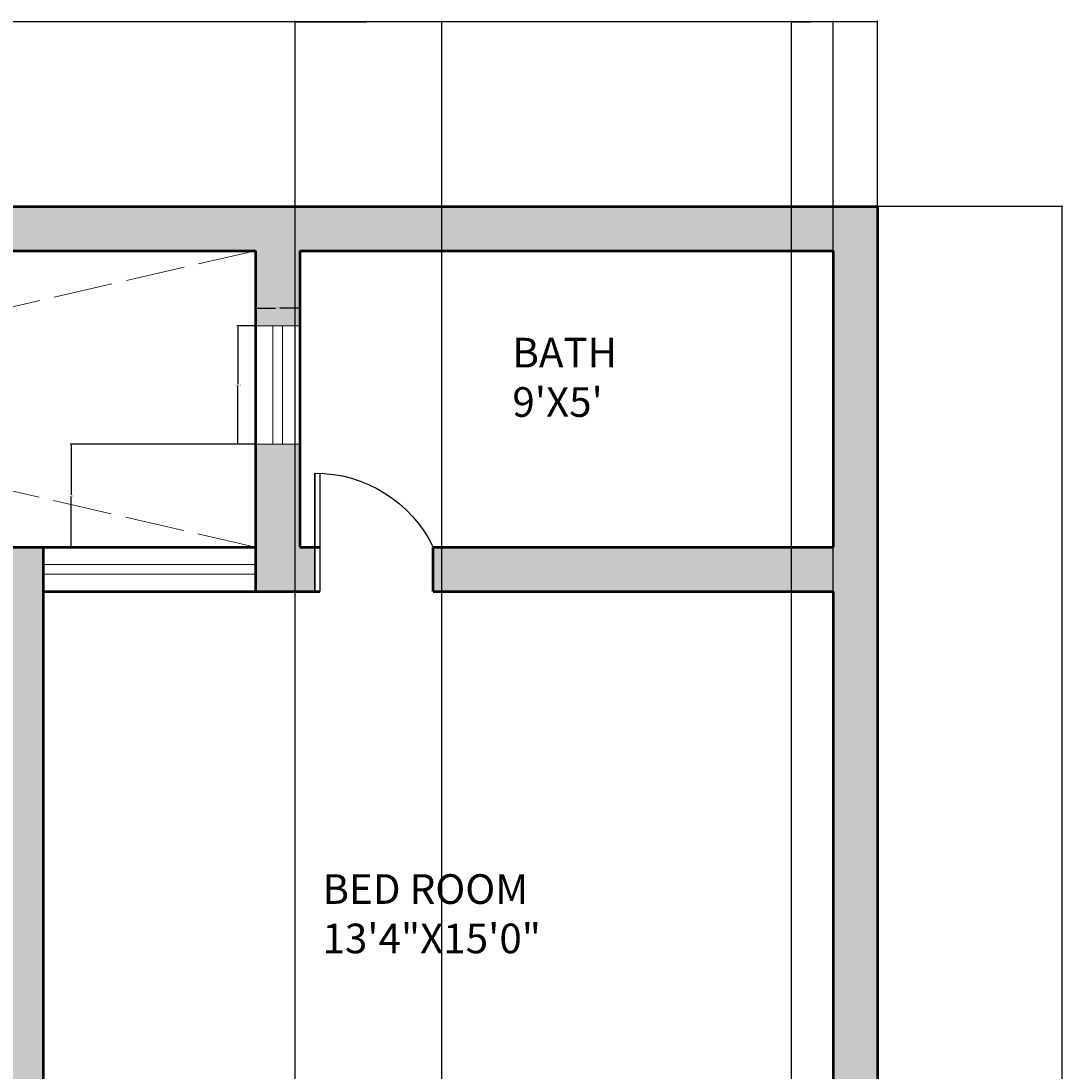
# Model space of a CAD drawing. Units: inches. Extents: x 383 to 970, y 275 to 1088.
# Tile 11 of 11: x 759 to 970, y 875 to 1088. Entities that reach past the tile are written whole.
import ezdxf

# ---------------------------------------------------------------- set-up
doc = ezdxf.new("R2010")
doc.units = ezdxf.units.IN
doc.header["$MEASUREMENT"] = 0
doc.linetypes.add('ACAD_ISO02W100', pattern=[15, 12, -3])
for name, color, linetype, lineweight in [('A-ANNO-DIMS', 2, 'Continuous', 18), ('A-AREA-IDEN', 7, 'Continuous', 18), ('A-DOOR', 3, 'Continuous', 25), ('A-FLOR-OPEN', 8, 'ACAD_ISO02W100', 13), ('A-GLAZ', 4, 'Continuous', 18), ('A-WALL', 7, 'Continuous', 50)]:
    doc.layers.add(name, color=color, linetype=linetype, lineweight=lineweight)
doc.layers.add('A-WALL-PATT', color=251, linetype='Continuous', lineweight=13, true_color=0x636466)
doc.styles.get("Standard").update_dxf_attribs({"font": 'arial.ttf'})
doc.dimstyles.get("Standard").update_dxf_attribs({"dimtxt": 0.18, "dimasz": 0.18, "dimexe": 0.18, "dimexo": 0.0625, "dimgap": 0.09, "dimtad": 0, "dimtih": 1, "dimtoh": 1, "dimdec": 4, "dimzin": 0, "dimdsep": 46, "dimtxsty": 'Standard', "dimcen": 0.09, "dimadec": 0, "dimazin": 0, "dimtfac": 1, "dimtdec": 4, "dimtofl": 0, "dimtmove": 0, "dimatfit": 3, "dimfxl": 1, "dimtolj": 1, "dimtzin": 0, "dimarcsym": 0})

# ---------------------------------------------------------------- blocks, each defined once
blk = doc.blocks.new('DOOR-LEAF-24IN')
for p, q in [((23, 24), (23, 0)), ((24, 0), (24, 24)), ((24, 0), (23, 0))]:
    blk.add_line(p, q)
blk.add_arc((24, -2.7), 26.7, 90, 154.0108)
blk = doc.blocks.new('WIN-VENT-24IN')
for p, q in [((0, 0), (0, 24)), ((3.5, 0), (3.5, 24)), ((5.5, 24), (5.5, 0)), ((9, 24), (9, 0))]:
    blk.add_line(p, q)
blk = doc.blocks.new('WIN-43IN')
for p, q in [((43, 9), (0, 9)), ((43, 5.5), (0, 5.5)), ((0, 3.5), (43, 3.5)), ((0, 0), (43, 0))]:
    blk.add_line(p, q)
blk = doc.blocks.new('*D19')
at = {"layer": 'A-ANNO-DIMS', "color": 0, "lineweight": -2, "transparency": 16777216}
for p, q in [((806.18, 1025.95), (802.46, 1025.95)), ((802.64, 1025.77), (802.64, 1014.13)), ((802.64, 1002.13), (802.64, 1013.77)), ((806.18, 1001.95), (802.46, 1001.95))]:
    blk.add_line(p, q, dxfattribs=at)
at = {"layer": 'A-ANNO-DIMS', "color": 0, "transparency": 16777216}
for points in [[(802.61, 1025.77), (802.67, 1025.77), (802.64, 1025.95)], [(802.61, 1002.13), (802.67, 1002.13), (802.64, 1001.95)]]:
    blk.add_solid(points, dxfattribs=at)
at = {"layer": 'Defpoints', "color": 0, "transparency": 16777216}
for p in [(806.24, 1025.95), (802.64, 1001.95), (806.24, 1001.95)]:
    blk.add_point(p, dxfattribs=at)
at = {"layer": 'A-ANNO-DIMS', "color": 0, "transparency": 16777216, "insert": (802.64, 1013.95), "char_height": 0.18, "attachment_point": 5}
blk.add_mtext('\\A1;VENT 24 TYP.', dxfattribs=at)
blk = doc.blocks.new('*D20')
at = {"layer": 'A-ANNO-DIMS', "color": 0, "lineweight": -2, "transparency": 16777216}
for p, q in [((806.24, 1026.01), (806.24, 1029.73)), ((806.42, 1029.55), (810.28, 1029.55)), ((815.06, 1029.55), (811.2, 1029.55)), ((815.24, 1026.01), (815.24, 1029.73))]:
    blk.add_line(p, q, dxfattribs=at)
at = {"layer": 'A-ANNO-DIMS', "color": 0, "transparency": 16777216}
for points in [[(806.42, 1029.58), (806.42, 1029.52), (806.24, 1029.55)], [(815.06, 1029.58), (815.06, 1029.52), (815.24, 1029.55)]]:
    blk.add_solid(points, dxfattribs=at)
at = {"layer": 'Defpoints', "color": 0, "transparency": 16777216}
for p in [(806.24, 1029.55), (806.24, 1025.95), (815.24, 1025.95)]:
    blk.add_point(p, dxfattribs=at)
at = {"layer": 'A-ANNO-DIMS', "color": 0, "transparency": 16777216, "insert": (810.74, 1029.55), "char_height": 0.18, "attachment_point": 5}
blk.add_mtext('\\A1;9 TYP.', dxfattribs=at)
blk = doc.blocks.new('*D37')
at = {"layer": 'A-ANNO-DIMS', "color": 0, "lineweight": -2, "transparency": 16777216}
for p, q in [((420.24, 1050.2), (420.24, 1087.67)), ((420.42, 1087.49), (675.95, 1087.49)), ((932.06, 1087.49), (676.53, 1087.49)), ((932.24, 1050.2), (932.24, 1087.67))]:
    blk.add_line(p, q, dxfattribs=at)
at = {"layer": 'A-ANNO-DIMS', "color": 0, "transparency": 16777216}
for points in [[(420.42, 1087.52), (420.42, 1087.46), (420.24, 1087.49)], [(932.06, 1087.52), (932.06, 1087.46), (932.24, 1087.49)]]:
    blk.add_solid(points, dxfattribs=at)
at = {"layer": 'Defpoints', "color": 0, "transparency": 16777216}
for p in [(932.24, 1087.49), (420.24, 1050.14), (932.24, 1050.14)]:
    blk.add_point(p, dxfattribs=at)
at = {"layer": 'A-ANNO-DIMS', "color": 0, "transparency": 16777216, "insert": (676.24, 1087.49), "char_height": 0.18, "attachment_point": 5}
blk.add_mtext('\\A1;512', dxfattribs=at)
blk = doc.blocks.new('*D38')
at = {"layer": 'A-ANNO-DIMS', "color": 0, "lineweight": -2, "transparency": 16777216}
for p, q in [((932.3, 1050.14), (969.77, 1050.14)), ((969.59, 1049.96), (969.59, 681.32)), ((969.59, 312.32), (969.59, 680.95)), ((932.3, 312.14), (969.77, 312.14))]:
    blk.add_line(p, q, dxfattribs=at)
at = {"layer": 'A-ANNO-DIMS', "color": 0, "transparency": 16777216}
for points in [[(969.56, 1049.96), (969.62, 1049.96), (969.59, 1050.14)], [(969.56, 312.32), (969.62, 312.32), (969.59, 312.14)]]:
    blk.add_solid(points, dxfattribs=at)
at = {"layer": 'Defpoints', "color": 0, "transparency": 16777216}
for p in [(932.24, 1050.14), (969.59, 1050.14), (932.24, 312.14)]:
    blk.add_point(p, dxfattribs=at)
at = {"layer": 'A-ANNO-DIMS', "color": 0, "transparency": 16777216, "insert": (969.59, 681.14), "char_height": 0.18, "attachment_point": 5}
blk.add_mtext('\\A1;738', dxfattribs=at)
blk = doc.blocks.new('*D59')
at = {"layer": 'A-ANNO-DIMS', "color": 0, "lineweight": -2, "transparency": 16777216}
for p, q in [((814.24, 645.02), (814.24, 1087.67)), ((814.42, 1087.49), (828.65, 1087.49)), ((843.8, 1087.49), (829.58, 1087.49)), ((843.98, 640.59), (843.98, 1087.67))]:
    blk.add_line(p, q, dxfattribs=at)
at = {"layer": 'A-ANNO-DIMS', "color": 0, "transparency": 16777216}
for points in [[(814.42, 1087.52), (814.42, 1087.46), (814.24, 1087.49)], [(843.8, 1087.52), (843.8, 1087.46), (843.98, 1087.49)]]:
    blk.add_solid(points, dxfattribs=at)
at = {"layer": 'Defpoints', "color": 0, "transparency": 16777216}
for p in [(814.24, 1087.49), (814.24, 644.96), (843.98, 640.52)]:
    blk.add_point(p, dxfattribs=at)
at = {"layer": 'A-ANNO-DIMS', "color": 0, "transparency": 16777216, "insert": (829.11, 1087.49), "char_height": 0.18, "attachment_point": 5}
blk.add_mtext('\\A1;29.744', dxfattribs=at)
blk = doc.blocks.new('*D61')
at = {"layer": 'A-ANNO-DIMS', "color": 0, "lineweight": -2, "transparency": 16777216}
for p, q in [((914.8, 712.66), (914.8, 1087.67)), ((914.98, 1087.49), (918.63, 1087.49)), ((923.06, 1087.49), (919.41, 1087.49)), ((923.24, 783.2), (923.24, 1087.67))]:
    blk.add_line(p, q, dxfattribs=at)
at = {"layer": 'A-ANNO-DIMS', "color": 0, "transparency": 16777216}
for points in [[(914.98, 1087.52), (914.98, 1087.46), (914.8, 1087.49)], [(923.06, 1087.52), (923.06, 1087.46), (923.24, 1087.49)]]:
    blk.add_solid(points, dxfattribs=at)
at = {"layer": 'Defpoints', "color": 0, "transparency": 16777216}
for p in [(923.24, 1087.49), (923.24, 783.14), (914.8, 712.6)]:
    blk.add_point(p, dxfattribs=at)
at = {"layer": 'A-ANNO-DIMS', "color": 0, "transparency": 16777216, "insert": (919.02, 1087.49), "char_height": 0.18, "attachment_point": 5}
blk.add_mtext('\\A1;8.439', dxfattribs=at)
blk = doc.blocks.new('*D63')
at = {"layer": 'A-ANNO-DIMS', "color": 0, "lineweight": -2, "transparency": 16777216}
for p, q in [((806.18, 1001.95), (768.71, 1001.95)), ((768.89, 1001.77), (768.89, 991.72)), ((768.89, 981.32), (768.89, 991.36)), ((806.18, 981.14), (768.71, 981.14))]:
    blk.add_line(p, q, dxfattribs=at)
at = {"layer": 'A-ANNO-DIMS', "color": 0, "transparency": 16777216}
for points in [[(768.86, 1001.77), (768.92, 1001.77), (768.89, 1001.95)], [(768.86, 981.32), (768.92, 981.32), (768.89, 981.14)]]:
    blk.add_solid(points, dxfattribs=at)
at = {"layer": 'Defpoints', "color": 0, "transparency": 16777216}
for p in [(768.89, 1001.95), (806.24, 1001.95), (806.24, 981.14)]:
    blk.add_point(p, dxfattribs=at)
at = {"layer": 'A-ANNO-DIMS', "color": 0, "transparency": 16777216, "insert": (768.89, 991.54), "char_height": 0.18, "attachment_point": 5}
blk.add_mtext('\\A1;20.813', dxfattribs=at)

msp = doc.modelspace()

# ---------------------------------------------------------------- hatches: boundary and pattern name
at = {"layer": 'A-WALL-PATT'}
h = msp.add_hatch(color=256, dxfattribs=at)
h.dxf.hatch_style = 1
h.paths.add_polyline_path([(651.24, 321.1365), (651.24, 417.1365), (735.24, 417.1365), (735.24, 491.9233), (726.24, 491.9233), (726.24, 426.1365), (582.24, 426.1365), (582.24, 606.1365), (687.24, 606.1365), (687.24, 615.1365), (573.24, 615.1365), (573.24, 546.1365), (570.24, 546.1365), (570.24, 537.1365), (573.24, 537.1365), (573.24, 414.1365), (582.24, 414.1365), (582.24, 417.1365), (642.24, 417.1365), (642.24, 321.1365), (621.6203, 321.1365), (621.6203, 312.1365), (651.24, 312.1365)], flags=17)
h.paths.add_polyline_path([(597.6203, 321.1365), (582.24, 321.1365), (582.24, 390.1365), (573.24, 390.1365), (573.24, 321.1365), (570.24, 321.1365), (570.24, 312.1365), (573.24, 312.1365), (597.6203, 312.1365)], flags=16)
h.paths.add_polyline_path([(534.24, 321.1365), (500.8868, 321.1365), (500.8868, 312.1365), (534.24, 312.1365)], flags=17)
h.paths.add_polyline_path([(735.24, 606.1365), (738.24, 606.1365), (738.24, 615.1365), (723.24, 615.1365), (723.24, 606.1365), (726.24, 606.1365), (726.24, 551.9233), (735.24, 551.9233)], flags=17)
h.paths.add_polyline_path([(848.0899, 615.1365), (814.24, 615.1365), (814.24, 689.38), (805.24, 689.38), (805.24, 615.1365), (802.24, 615.1365), (802.24, 606.1365), (848.0899, 606.1365)], flags=17)
h.paths.add_polyline_path([(530.24, 615.1365), (498.24, 615.1365), (498.24, 646.5351), (489.24, 646.5351), (489.24, 615.1365), (466.771, 615.1365), (466.771, 606.1365), (521.24, 606.1365), (521.24, 603.1365), (530.24, 603.1365), (530.24, 606.1365)], flags=17)
h.paths.add_polyline_path([(498.24, 744.1365), (489.24, 744.1365), (489.24, 706.5351), (498.24, 706.5351)], flags=17)
h.paths.add_polyline_path([(715.24, 792.1365), (598.24, 792.1365), (598.24, 972.1365), (636.5058, 972.1365), (636.5058, 981.1365), (589.24, 981.1365), (589.24, 972.1365), (589.24, 792.1365), (586.24, 792.1365), (586.24, 783.1365), (589.24, 783.1365), (715.24, 783.1365)], flags=17)
h.paths.add_polyline_path([(763.24, 981.1365), (696.5058, 981.1365), (696.5058, 972.1365), (754.24, 972.1365), (754.24, 792.1365), (751.24, 792.1365), (751.24, 783.1365), (754.24, 783.1365), (764.24, 783.1365), (764.24, 792.1365), (763.24, 792.1365)], flags=17)
h.paths.add_polyline_path([(815.24, 1001.9492), (806.24, 1001.9492), (806.24, 972.1365), (818.24, 972.1365), (818.24, 981.1365), (815.24, 981.1365)], flags=17)
h.paths.add_polyline_path([(546.24, 1004.0336), (537.24, 1004.0336), (537.24, 981.1365), (534.24, 981.1365), (534.24, 972.1365), (537.24, 972.1365), (546.24, 972.1365), (546.24, 981.1365)], flags=17)
h.paths.add_polyline_path([(884.0899, 606.1365), (932.24, 606.1365), (932.24, 1050.1365), (420.24, 1050.1365), (420.24, 312.1365), (440.8868, 312.1365), (440.8868, 321.1365), (429.24, 321.1365), (429.24, 537.1365), (538.24, 537.1365), (538.24, 546.1365), (530.24, 546.1365), (530.24, 579.1365), (521.24, 579.1365), (521.24, 546.1365), (429.24, 546.1365), (429.24, 606.1365), (442.771, 606.1365), (442.771, 615.1365), (429.24, 615.1365), (429.24, 783.1365), (489.24, 783.1365), (489.24, 780.1365), (498.24, 780.1365), (498.24, 783.1365), (550.24, 783.1365), (550.24, 792.1365), (429.24, 792.1365), (429.24, 972.1365), (510.24, 972.1365), (510.24, 981.1365), (429.24, 981.1365), (429.24, 1041.1365), (537.24, 1041.1365), (537.24, 1028.0336), (546.24, 1028.0336), (546.24, 1041.1365), (806.24, 1041.1365), (806.24, 1025.9492), (815.24, 1025.9492), (815.24, 1041.1365), (923.24, 1041.1365), (923.24, 981.1365), (842.24, 981.1365), (842.24, 972.1365), (923.24, 972.1365), (923.24, 792.1365), (800.24, 792.1365), (800.24, 783.1365), (805.24, 783.1365), (805.24, 725.38), (814.24, 725.38), (814.24, 783.1365), (923.24, 783.1365), (923.24, 615.1365), (884.0899, 615.1365)])

# ---------------------------------------------------------------- linework, layer by layer
at = {"layer": 'A-DOOR'}
msp.add_line((818.24, 996.1365), (818.24, 972.1365), dxfattribs=at)
at = {"layer": 'A-FLOR-OPEN'}
for p, q in [((546.24, 981.1365), (806.24, 1041.1365)), ((806.24, 981.1365), (546.24, 1041.1365))]:
    msp.add_line(p, q, dxfattribs=at)
at = {"layer": 'A-GLAZ'}
for p, q in [((806.24, 1025.9492), (815.24, 1025.9492)), ((815.24, 1001.9492), (806.24, 1001.9492)), ((763.24, 981.1365), (763.24, 972.1365)), ((806.24, 972.1365), (806.24, 981.1365))]:
    msp.add_line(p, q, dxfattribs=at)
at = {"layer": 'A-WALL'}
for p, q in [((420.24, 1050.1365), (932.24, 1050.1365)), ((932.24, 1050.1365), (932.24, 312.1365)), ((546.24, 1041.1365), (806.24, 1041.1365)), ((806.24, 1041.1365), (806.24, 972.1365)), ((815.24, 1041.1365), (815.24, 981.1365)), ((815.24, 1041.1365), (923.24, 1041.1365)), ((923.24, 1041.1365), (923.24, 981.1365)), ((546.24, 981.1365), (806.24, 981.1365)), ((763.24, 981.1365), (763.24, 792.1365)), ((815.24, 981.1365), (819.24, 981.1365)), ((842.24, 972.1365), (842.24, 981.1365)), ((842.24, 981.1365), (923.24, 981.1365)), ((763.24, 972.1365), (819.24, 972.1365)), ((815.24, 972.1365), (818.24, 972.1365)), ((842.24, 972.1365), (923.24, 972.1365)), ((923.24, 972.1365), (923.24, 792.1365))]:
    msp.add_line(p, q, dxfattribs=at)

# ---------------------------------------------------------------- block references
at = {"layer": 'A-DOOR', "extrusion": (0, 0, -1), "zscale": -1}
msp.add_blockref('DOOR-LEAF-24IN', (-842.2401, 972.136), dxfattribs=at)
at = {"layer": 'A-GLAZ', "rotation": 180}
for name, p in [('WIN-VENT-24IN', (815.2401, 1025.9488)), ('WIN-43IN', (806.2401, 981.137))]:
    msp.add_blockref(name, p, dxfattribs=at)

# ---------------------------------------------------------------- texts
at = {"layer": 'A-AREA-IDEN', "char_height": 6, "attachment_point": 1}
for s, width, insert in [("BATH\\P9'X5'", 46.963316, (858.2635, 1023.5193)), ('BED ROOM\\P13\'4"X15\'0"', 65.973353, (819.7958, 914.8987))]:
    msp.add_mtext_dynamic_manual_height_columns(s, width=width, gutter_width=30, heights=[0], dxfattribs=dict(at, insert=insert))

# ---------------------------------------------------------------- dimensions: what is measured, and where the dimension line sits
at = {"layer": 'A-ANNO-DIMS'}
for base, p1, p2, override, picture, middle in [((932.24, 1087.4865), (420.24, 1050.1365), (932.24, 1050.1365), {"dimdec": 0, "dimlfac": 1, "dimrnd": 0, "dimzin": 0, "dimdsep": 46, "dimlunit": 2}, '*D37', (676.24, 1087.4865)), ((814.24, 1087.4865), (843.9841, 640.5231), (814.24, 644.9565), {"dimdec": 3, "dimlfac": 1, "dimrnd": 0, "dimzin": 0, "dimdsep": 46, "dimlunit": 2}, '*D59', (829.1121, 1087.4865)), ((923.24, 1087.4865), (914.8009, 712.601), (923.24, 783.1365), {"dimdec": 3, "dimlfac": 1, "dimrnd": 0, "dimzin": 0, "dimdsep": 46, "dimlunit": 2}, '*D61', (919.0205, 1087.4865))]:
    dim = msp.add_linear_dim(base=base, p1=p1, p2=p2, dimstyle='Standard', override=override, dxfattribs=at)
    dim.commit()
    dim.dimension.update_dxf_attribs({"geometry": picture, "text_midpoint": middle})
for base, p1, p2, override, picture, middle in [((969.59, 1050.1365), (932.24, 312.1365), (932.24, 1050.1365), {"dimdec": 0, "dimlfac": 1, "dimrnd": 0, "dimzin": 0, "dimdsep": 46, "dimlunit": 2}, '*D38', (969.59, 681.1365)), ((768.89, 1001.9492), (806.24, 981.1365), (806.24, 1001.9492), {"dimdec": 3, "dimlfac": 1, "dimrnd": 0, "dimzin": 0, "dimdsep": 46, "dimlunit": 2}, '*D63', (768.89, 991.5428))]:
    dim = msp.add_linear_dim(base=base, p1=p1, p2=p2, angle=90, dimstyle='Standard', override=override, dxfattribs=at)
    dim.commit()
    dim.dimension.update_dxf_attribs({"geometry": picture, "text_midpoint": middle})
for base, p1, p2, angle, text, picture, middle in [((806.24, 1029.5492), (815.24, 1025.9492), (806.24, 1025.9492), 180, '<> TYP.', '*D20', (810.74, 1029.5492)), ((802.64, 1001.9492), (806.24, 1025.9492), (806.24, 1001.9492), 270, 'VENT <> TYP.', '*D19', (802.64, 1013.9492))]:
    dim = msp.add_linear_dim(base=base, p1=p1, p2=p2, angle=angle, text=text, dimstyle='Standard', override={"dimdec": 0, "dimlfac": 1, "dimrnd": 0, "dimzin": 0, "dimdsep": 46, "dimlunit": 2}, dxfattribs=at)
    dim.commit()
    dim.dimension.update_dxf_attribs({"geometry": picture, "text_midpoint": middle})

doc.saveas('drawing.dxf')
